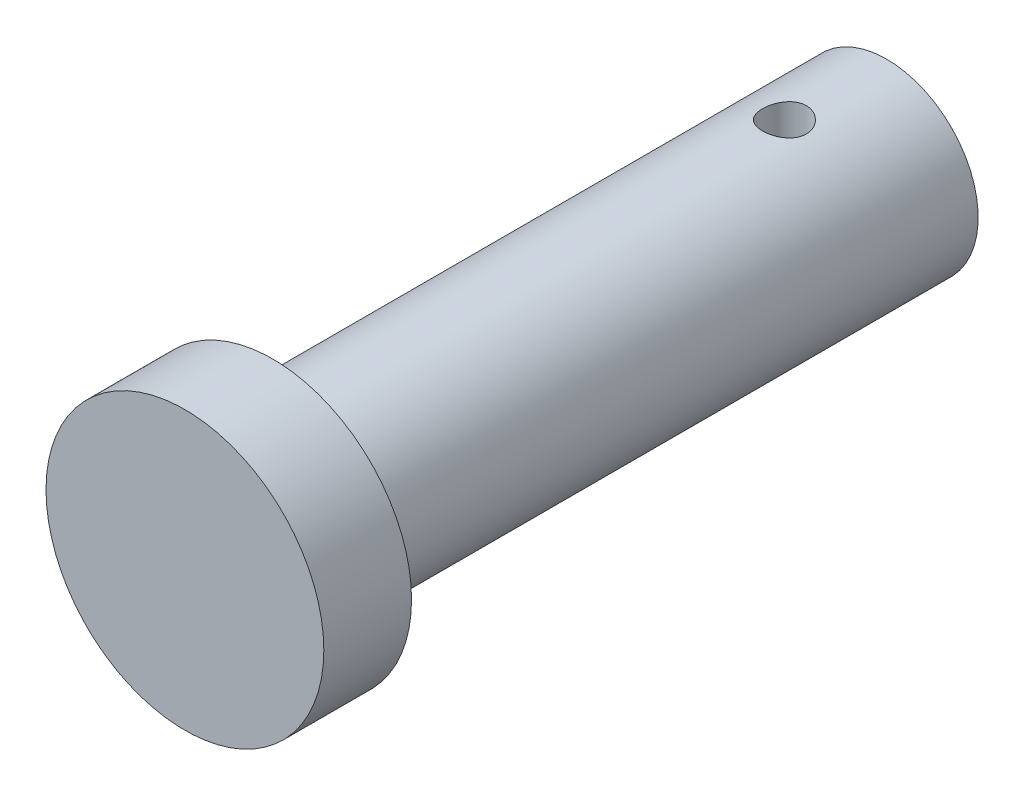
ISO-10303-21;
HEADER;
FILE_DESCRIPTION(('STEP AP214'),'2;1');
FILE_NAME('part.step','',(''),(''),'','','');
FILE_SCHEMA(('AUTOMOTIVE_DESIGN { 1 0 10303 214 1 1 1 1 }'));
ENDSEC;
DATA;
#1=APPLICATION_CONTEXT('core data for automotive mechanical design processes');
#2=APPLICATION_PROTOCOL_DEFINITION('international standard','automotive_design',2000,#1);
#3=PRODUCT_CONTEXT('',#1,'mechanical');
#4=PRODUCT('Part','Part','',(#3));
#5=PRODUCT_RELATED_PRODUCT_CATEGORY('part','',(#4));
#6=PRODUCT_DEFINITION_FORMATION('','',#4);
#7=PRODUCT_DEFINITION_CONTEXT('part definition',#1,'design');
#8=PRODUCT_DEFINITION('design','',#6,#7);
#9=PRODUCT_DEFINITION_SHAPE('','',#8);
#10=(LENGTH_UNIT() NAMED_UNIT(*) SI_UNIT(.MILLI.,.METRE.));
#11=(NAMED_UNIT(*) PLANE_ANGLE_UNIT() SI_UNIT($,.RADIAN.));
#12=(NAMED_UNIT(*) SI_UNIT($,.STERADIAN.) SOLID_ANGLE_UNIT());
#13=UNCERTAINTY_MEASURE_WITH_UNIT(LENGTH_MEASURE(1.E-05),#10,'distance_accuracy_value','');
#14=(GEOMETRIC_REPRESENTATION_CONTEXT(3) GLOBAL_UNCERTAINTY_ASSIGNED_CONTEXT((#13)) GLOBAL_UNIT_ASSIGNED_CONTEXT((#10,
#11,#12)) REPRESENTATION_CONTEXT('',''));
#15=CARTESIAN_POINT('',(0.,0.,0.));
#16=DIRECTION('',(0.,0.,1.));
#17=DIRECTION('',(1.,0.,0.));
#18=AXIS2_PLACEMENT_3D('',#15,#16,#17);
#19=CARTESIAN_POINT('',(0.,0.,12.));
#20=DIRECTION('',(0.,0.,-1.));
#21=DIRECTION('',(-1.,0.,0.));
#22=AXIS2_PLACEMENT_3D('',#19,#20,#21);
#23=CYLINDRICAL_SURFACE('',#22,19.);
#24=CARTESIAN_POINT('',(0.,0.,12.));
#25=DIRECTION('',(0.,0.,1.));
#26=DIRECTION('',(1.,0.,0.));
#27=AXIS2_PLACEMENT_3D('',#24,#25,#26);
#28=CIRCLE('',#27,19.);
#29=CARTESIAN_POINT('',(19.,0.,12.));
#30=VERTEX_POINT('',#29);
#31=EDGE_CURVE('E47',#30,#30,#28,.T.);
#32=ORIENTED_EDGE('',*,*,#31,.F.);
#33=EDGE_LOOP('',(#32));
#34=FACE_BOUND('',#33,.T.);
#35=CARTESIAN_POINT('',(0.,0.,0.));
#36=DIRECTION('',(0.,0.,1.));
#37=DIRECTION('',(1.,0.,0.));
#38=AXIS2_PLACEMENT_3D('',#35,#36,#37);
#39=CIRCLE('',#38,19.);
#40=CARTESIAN_POINT('',(19.,0.,0.));
#41=VERTEX_POINT('',#40);
#42=EDGE_CURVE('E53',#41,#41,#39,.T.);
#43=ORIENTED_EDGE('',*,*,#42,.T.);
#44=EDGE_LOOP('',(#43));
#45=FACE_BOUND('',#44,.T.);
#46=ADVANCED_FACE('F40',(#34,#45),#23,.T.);
#47=CARTESIAN_POINT('',(0.,0.,12.));
#48=DIRECTION('',(0.,0.,1.));
#49=DIRECTION('',(1.,0.,0.));
#50=AXIS2_PLACEMENT_3D('',#47,#48,#49);
#51=PLANE('',#50);
#52=ORIENTED_EDGE('',*,*,#31,.T.);
#53=EDGE_LOOP('',(#52));
#54=FACE_BOUND('',#53,.T.);
#55=ADVANCED_FACE('F83',(#54),#51,.T.);
#56=CARTESIAN_POINT('',(0.,0.,0.));
#57=DIRECTION('',(0.,0.,1.));
#58=DIRECTION('',(1.,0.,0.));
#59=AXIS2_PLACEMENT_3D('',#56,#57,#58);
#60=PLANE('',#59);
#61=CARTESIAN_POINT('',(0.,0.,0.));
#62=DIRECTION('',(0.,0.,-1.));
#63=DIRECTION('',(-1.,0.,0.));
#64=AXIS2_PLACEMENT_3D('',#61,#62,#63);
#65=CIRCLE('',#64,12.5);
#66=CARTESIAN_POINT('',(-12.5,0.,0.));
#67=VERTEX_POINT('',#66);
#68=EDGE_CURVE('E10',#67,#67,#65,.T.);
#69=ORIENTED_EDGE('',*,*,#68,.F.);
#70=EDGE_LOOP('',(#69));
#71=FACE_BOUND('',#70,.T.);
#72=ORIENTED_EDGE('',*,*,#42,.F.);
#73=EDGE_LOOP('',(#72));
#74=FACE_BOUND('',#73,.T.);
#75=ADVANCED_FACE('F82',(#71,#74),#60,.F.);
#76=CARTESIAN_POINT('',(0.,0.,-84.));
#77=DIRECTION('',(0.,0.,1.));
#78=DIRECTION('',(1.,0.,0.));
#79=AXIS2_PLACEMENT_3D('',#76,#77,#78);
#80=CYLINDRICAL_SURFACE('',#79,12.5);
#81=CARTESIAN_POINT('',(0.,-12.5,-67.));
#82=CARTESIAN_POINT('',(0.165963929028719,-12.4999970714968,-67.0000050240773));
#83=CARTESIAN_POINT('',(0.331985420928071,-12.4966615634859,-67.0138184102361));
#84=CARTESIAN_POINT('',(0.659284290971384,-12.4836783946933,-67.0686327395954));
#85=CARTESIAN_POINT('',(0.820558683214278,-12.4740268462166,-67.1096504279947));
#86=CARTESIAN_POINT('',(1.13358839471402,-12.4494823208195,-67.2174923345044));
#87=CARTESIAN_POINT('',(1.28535442324823,-12.4345953702841,-67.2842868898576));
#88=CARTESIAN_POINT('',(1.57552517879764,-12.4011725442513,-67.4416854364459));
#89=CARTESIAN_POINT('',(1.71392971475167,-12.3826366165873,-67.5322897680773));
#90=CARTESIAN_POINT('',(1.97609263393973,-12.3435386014785,-67.7365641783755));
#91=CARTESIAN_POINT('',(2.0995595210048,-12.3229472454311,-67.8506027810493));
#92=CARTESIAN_POINT('',(2.32581080811943,-12.2822574370147,-68.0977188690646));
#93=CARTESIAN_POINT('',(2.4285930462449,-12.2621590363612,-68.230798342041));
#94=CARTESIAN_POINT('',(2.61189993555015,-12.224437969062,-68.5144458330174));
#95=CARTESIAN_POINT('',(2.69210377047565,-12.2068525815312,-68.6652265837588));
#96=CARTESIAN_POINT('',(2.82591582947333,-12.1765733412448,-68.9786198351285));
#97=CARTESIAN_POINT('',(2.87952794169564,-12.1638787734309,-69.1412306020232));
#98=CARTESIAN_POINT('',(2.95765058108664,-12.1451184675007,-69.4704765732689));
#99=CARTESIAN_POINT('',(2.98268262400617,-12.1389341034343,-69.6369811215255));
#100=CARTESIAN_POINT('',(3.00455808879087,-12.1335389605945,-69.9719323796428));
#101=CARTESIAN_POINT('',(3.001405716824,-12.1343271412568,-70.1403787959569));
#102=CARTESIAN_POINT('',(2.96741912081943,-12.1426811387008,-70.4704759660129));
#103=CARTESIAN_POINT('',(2.93720103400495,-12.1500960921292,-70.6321945651895));
#104=CARTESIAN_POINT('',(2.85092141637189,-12.1706283738785,-70.9481973166478));
#105=CARTESIAN_POINT('',(2.79485817372028,-12.1837460799133,-71.1024809757344));
#106=CARTESIAN_POINT('',(2.65794121231782,-12.2143476734445,-71.4009129780844));
#107=CARTESIAN_POINT('',(2.5768594824696,-12.2318714325758,-71.5449524529167));
#108=CARTESIAN_POINT('',(2.39236688956382,-12.2692875046197,-71.8176045007226));
#109=CARTESIAN_POINT('',(2.28895240342647,-12.2891802016137,-71.9462145652851));
#110=CARTESIAN_POINT('',(2.05951493908847,-12.329732025739,-72.1878935703187));
#111=CARTESIAN_POINT('',(1.93297064389908,-12.3503975788014,-72.3004670990622));
#112=CARTESIAN_POINT('',(1.66255592459692,-12.3896951594929,-72.5028847197464));
#113=CARTESIAN_POINT('',(1.51868504982141,-12.4083271342049,-72.5927282202926));
#114=CARTESIAN_POINT('',(1.21702847718581,-12.4415394956922,-72.7472972206128));
#115=CARTESIAN_POINT('',(1.05920278696055,-12.4561077058019,-72.8119474562378));
#116=CARTESIAN_POINT('',(0.734497606078676,-12.4794620474154,-72.9136650790486));
#117=CARTESIAN_POINT('',(0.56761971338766,-12.4882491958651,-72.9507373176268));
#118=CARTESIAN_POINT('',(0.233787399651661,-12.4989027542709,-72.9955020646521));
#119=CARTESIAN_POINT('',(0.0669284805450053,-12.5009282130753,-73.0038698924616));
#120=CARTESIAN_POINT('',(-0.26580438158663,-12.4982807419474,-72.9928332331491));
#121=CARTESIAN_POINT('',(-0.431678404764951,-12.4936083648176,-72.9734310380128));
#122=CARTESIAN_POINT('',(-0.755422580108846,-12.4781916395217,-72.9079630214836));
#123=CARTESIAN_POINT('',(-0.913370579311304,-12.4675301590363,-72.8622608904262));
#124=CARTESIAN_POINT('',(-1.21935330013476,-12.4413335015664,-72.7459018083048));
#125=CARTESIAN_POINT('',(-1.3673870666415,-12.4257978558334,-72.6752424570219));
#126=CARTESIAN_POINT('',(-1.6520615099557,-12.3911910149582,-72.5096334064021));
#127=CARTESIAN_POINT('',(-1.78847176740356,-12.3720653178033,-72.4142992830756));
#128=CARTESIAN_POINT('',(-2.04359904096633,-12.3324936406987,-72.2025430709866));
#129=CARTESIAN_POINT('',(-2.16231325074337,-12.3120474520734,-72.0861176439192));
#130=CARTESIAN_POINT('',(-2.38142453789941,-12.2715742142771,-71.8323591687915));
#131=CARTESIAN_POINT('',(-2.48134974047369,-12.2515669262668,-71.6946148779179));
#132=CARTESIAN_POINT('',(-2.65666020824081,-12.2147538797452,-71.4039095721033));
#133=CARTESIAN_POINT('',(-2.7320465722335,-12.1979479778962,-71.2509492389065));
#134=CARTESIAN_POINT('',(-2.85558993518171,-12.1696189519335,-70.934987486456));
#135=CARTESIAN_POINT('',(-2.90390754385905,-12.1580647463107,-70.7720517965788));
#136=CARTESIAN_POINT('',(-2.97238380283979,-12.1415072663683,-70.4400538149793));
#137=CARTESIAN_POINT('',(-2.99254804274991,-12.1365026916888,-70.2709927462382));
#138=CARTESIAN_POINT('',(-3.00387066449353,-12.1337046220624,-69.9363292997194));
#139=CARTESIAN_POINT('',(-2.99578106592266,-12.1357241633848,-69.7707535036733));
#140=CARTESIAN_POINT('',(-2.95253345626267,-12.1463176460425,-69.4434002357763));
#141=CARTESIAN_POINT('',(-2.91737590900096,-12.1548914750658,-69.2816226988886));
#142=CARTESIAN_POINT('',(-2.82138591303537,-12.1775274976748,-68.9672024474518));
#143=CARTESIAN_POINT('',(-2.76068402045611,-12.191561756094,-68.8145177274163));
#144=CARTESIAN_POINT('',(-2.61543373580582,-12.2235433612686,-68.5213955861163));
#145=CARTESIAN_POINT('',(-2.53088229934855,-12.2414912075257,-68.3809597314136));
#146=CARTESIAN_POINT('',(-2.33793007708463,-12.279819325529,-68.1126629998805));
#147=CARTESIAN_POINT('',(-2.22900267979018,-12.3002478697533,-67.9851876769013));
#148=CARTESIAN_POINT('',(-1.99143074773236,-12.3409359831145,-67.7500800119481));
#149=CARTESIAN_POINT('',(-1.86278158874233,-12.361195511444,-67.6424523367898));
#150=CARTESIAN_POINT('',(-1.58688299880139,-12.3996570299581,-67.4483907404453));
#151=CARTESIAN_POINT('',(-1.43936414359401,-12.4178200201219,-67.362331594558));
#152=CARTESIAN_POINT('',(-1.13153622828567,-12.4496380610582,-67.2163704672521));
#153=CARTESIAN_POINT('',(-0.971236973691219,-12.4632965272855,-67.1564486566084));
#154=CARTESIAN_POINT('',(-0.675887025694763,-12.4824059901497,-67.0739613748622));
#155=CARTESIAN_POINT('',(-0.542312066268418,-12.4889599449579,-67.0462833842143));
#156=CARTESIAN_POINT('',(-0.272504227478245,-12.4977580149525,-67.0093012191481));
#157=CARTESIAN_POINT('',(-0.136271517915773,-12.5000024045682,-66.9999958747745));
#158=CARTESIAN_POINT('',(0.,-12.5,-67.));
#159=B_SPLINE_CURVE_WITH_KNOTS('',3,(#81,#82,#83,#84,#85,#86,#87,#88,#89,#90,#91,#92,#93,#94,
#95,#96,#97,#98,#99,#100,#101,#102,#103,#104,#105,#106,#107,#108,#109,#110,#111,#112,#113,#114,
#115,#116,#117,#118,#119,#120,#121,#122,#123,#124,#125,#126,#127,#128,#129,#130,#131,#132,#133,
#134,#135,#136,#137,#138,#139,#140,#141,#142,#143,#144,#145,#146,#147,#148,#149,#150,#151,#152,
#153,#154,#155,#156,#157,#158),.UNSPECIFIED.,.T.,.F.,(4,2,2,2,2,2,2,2,2,2,2,2,2,2,2,2,2,2,2,2,2,
2,2,2,2,2,2,2,2,2,2,2,2,2,2,2,2,2,4),(0.,0.497392599366679,0.995091645758826,1.49221966408501,
1.9893547899852,2.49500570148357,3.00070943533306,3.51327262050848,4.02576083835037,
4.52873995359112,5.03164400680464,5.52338274964838,6.01515406709139,6.51154667521173,
7.00801987450004,7.51749958381935,8.02699254752171,8.53799614678204,9.04890983140416,
9.54771776810827,10.0464845383097,10.5385143736981,11.0305915421211,11.5308523313794,
12.0311923705731,12.5427824523192,13.0543496229378,13.5628484119093,14.0712462285019,
14.5662165454702,15.0611783809799,15.5536406351284,16.0461657803879,16.5505844610431,
17.055121595827,17.5678974206352,18.0802835459069,18.4887142303991,18.897118905514),.UNSPECIFIED.);
#160=CARTESIAN_POINT('',(0.,-12.5,-67.));
#161=VERTEX_POINT('',#160);
#162=EDGE_CURVE('E37',#161,#161,#159,.T.);
#163=ORIENTED_EDGE('',*,*,#162,.T.);
#164=EDGE_LOOP('',(#163));
#165=FACE_BOUND('',#164,.T.);
#166=CARTESIAN_POINT('',(0.,12.5,-67.));
#167=CARTESIAN_POINT('',(-0.165963929028713,12.4999970714968,-67.0000050240773));
#168=CARTESIAN_POINT('',(-0.331985420928065,12.4966615634859,-67.0138184102361));
#169=CARTESIAN_POINT('',(-0.659284290971378,12.4836783946932,-67.0686327395954));
#170=CARTESIAN_POINT('',(-0.820558683214273,12.4740268462166,-67.1096504279947));
#171=CARTESIAN_POINT('',(-1.13358839471402,12.4494823208195,-67.2174923345044));
#172=CARTESIAN_POINT('',(-1.28535442324822,12.4345953702841,-67.2842868898576));
#173=CARTESIAN_POINT('',(-1.57552517879763,12.4011725442513,-67.4416854364459));
#174=CARTESIAN_POINT('',(-1.71392971475166,12.3826366165873,-67.5322897680773));
#175=CARTESIAN_POINT('',(-1.97609263393972,12.3435386014785,-67.7365641783755));
#176=CARTESIAN_POINT('',(-2.0995595210048,12.3229472454311,-67.8506027810493));
#177=CARTESIAN_POINT('',(-2.32581080811943,12.2822574370147,-68.0977188690646));
#178=CARTESIAN_POINT('',(-2.42859304624489,12.2621590363612,-68.230798342041));
#179=CARTESIAN_POINT('',(-2.61189993555015,12.224437969062,-68.5144458330175));
#180=CARTESIAN_POINT('',(-2.69210377047565,12.2068525815312,-68.6652265837589));
#181=CARTESIAN_POINT('',(-2.82591582947333,12.1765733412448,-68.9786198351285));
#182=CARTESIAN_POINT('',(-2.87952794169564,12.1638787734309,-69.1412306020232));
#183=CARTESIAN_POINT('',(-2.95765058108663,12.1451184675007,-69.4704765732689));
#184=CARTESIAN_POINT('',(-2.98268262400616,12.1389341034343,-69.6369811215255));
#185=CARTESIAN_POINT('',(-3.00455808879087,12.1335389605945,-69.9719323796428));
#186=CARTESIAN_POINT('',(-3.00140571682399,12.1343271412568,-70.1403787959569));
#187=CARTESIAN_POINT('',(-2.96741912081942,12.1426811387008,-70.4704759660129));
#188=CARTESIAN_POINT('',(-2.93720103400494,12.1500960921292,-70.6321945651895));
#189=CARTESIAN_POINT('',(-2.85092141637189,12.1706283738785,-70.9481973166478));
#190=CARTESIAN_POINT('',(-2.79485817372027,12.1837460799133,-71.1024809757344));
#191=CARTESIAN_POINT('',(-2.65794121231781,12.2143476734445,-71.4009129780844));
#192=CARTESIAN_POINT('',(-2.57685948246959,12.2318714325758,-71.5449524529167));
#193=CARTESIAN_POINT('',(-2.39236688956382,12.2692875046197,-71.8176045007226));
#194=CARTESIAN_POINT('',(-2.28895240342646,12.2891802016137,-71.9462145652851));
#195=CARTESIAN_POINT('',(-2.05951493908846,12.329732025739,-72.1878935703187));
#196=CARTESIAN_POINT('',(-1.93297064389908,12.3503975788014,-72.3004670990622));
#197=CARTESIAN_POINT('',(-1.66255592459691,12.3896951594929,-72.5028847197464));
#198=CARTESIAN_POINT('',(-1.5186850498214,12.4083271342049,-72.5927282202926));
#199=CARTESIAN_POINT('',(-1.21702847718581,12.4415394956922,-72.7472972206128));
#200=CARTESIAN_POINT('',(-1.05920278696054,12.4561077058019,-72.8119474562378));
#201=CARTESIAN_POINT('',(-0.734497606078672,12.4794620474154,-72.9136650790486));
#202=CARTESIAN_POINT('',(-0.567619713387655,12.4882491958651,-72.9507373176268));
#203=CARTESIAN_POINT('',(-0.233787399651657,12.4989027542709,-72.9955020646521));
#204=CARTESIAN_POINT('',(-0.0669284805450011,12.5009282130753,-73.0038698924616));
#205=CARTESIAN_POINT('',(0.265804381586634,12.4982807419474,-72.9928332331491));
#206=CARTESIAN_POINT('',(0.431678404764957,12.4936083648176,-72.9734310380128));
#207=CARTESIAN_POINT('',(0.75542258010885,12.4781916395217,-72.9079630214836));
#208=CARTESIAN_POINT('',(0.913370579311307,12.4675301590363,-72.8622608904262));
#209=CARTESIAN_POINT('',(1.21935330013476,12.4413335015664,-72.7459018083048));
#210=CARTESIAN_POINT('',(1.3673870666415,12.4257978558334,-72.6752424570219));
#211=CARTESIAN_POINT('',(1.65206150995571,12.3911910149582,-72.5096334064021));
#212=CARTESIAN_POINT('',(1.78847176740356,12.3720653178033,-72.4142992830756));
#213=CARTESIAN_POINT('',(2.04359904096634,12.3324936406987,-72.2025430709866));
#214=CARTESIAN_POINT('',(2.16231325074337,12.3120474520734,-72.0861176439192));
#215=CARTESIAN_POINT('',(2.38142453789941,12.2715742142771,-71.8323591687915));
#216=CARTESIAN_POINT('',(2.4813497404737,12.2515669262668,-71.6946148779179));
#217=CARTESIAN_POINT('',(2.65666020824082,12.2147538797452,-71.4039095721033));
#218=CARTESIAN_POINT('',(2.7320465722335,12.1979479778962,-71.2509492389065));
#219=CARTESIAN_POINT('',(2.85558993518172,12.1696189519335,-70.934987486456));
#220=CARTESIAN_POINT('',(2.90390754385905,12.1580647463107,-70.7720517965788));
#221=CARTESIAN_POINT('',(2.97238380283979,12.1415072663683,-70.4400538149793));
#222=CARTESIAN_POINT('',(2.99254804274991,12.1365026916888,-70.2709927462382));
#223=CARTESIAN_POINT('',(3.00387066449354,12.1337046220624,-69.9363292997194));
#224=CARTESIAN_POINT('',(2.99578106592266,12.1357241633848,-69.7707535036733));
#225=CARTESIAN_POINT('',(2.95253345626268,12.1463176460425,-69.4434002357763));
#226=CARTESIAN_POINT('',(2.91737590900097,12.1548914750658,-69.2816226988886));
#227=CARTESIAN_POINT('',(2.82138591303538,12.1775274976748,-68.9672024474518));
#228=CARTESIAN_POINT('',(2.76068402045612,12.191561756094,-68.8145177274163));
#229=CARTESIAN_POINT('',(2.61543373580584,12.2235433612686,-68.5213955861163));
#230=CARTESIAN_POINT('',(2.53088229934856,12.2414912075257,-68.3809597314137));
#231=CARTESIAN_POINT('',(2.33793007708465,12.279819325529,-68.1126629998805));
#232=CARTESIAN_POINT('',(2.2290026797902,12.3002478697533,-67.9851876769013));
#233=CARTESIAN_POINT('',(1.99143074773238,12.3409359831145,-67.7500800119481));
#234=CARTESIAN_POINT('',(1.86278158874235,12.361195511444,-67.6424523367898));
#235=CARTESIAN_POINT('',(1.58688299880141,12.3996570299581,-67.4483907404453));
#236=CARTESIAN_POINT('',(1.43936414359403,12.4178200201219,-67.362331594558));
#237=CARTESIAN_POINT('',(1.13153622828568,12.4496380610582,-67.2163704672521));
#238=CARTESIAN_POINT('',(0.971236973691228,12.4632965272855,-67.1564486566084));
#239=CARTESIAN_POINT('',(0.675887025694771,12.4824059901497,-67.0739613748622));
#240=CARTESIAN_POINT('',(0.542312066268425,12.4889599449579,-67.0462833842143));
#241=CARTESIAN_POINT('',(0.272504227478252,12.4977580149525,-67.0093012191481));
#242=CARTESIAN_POINT('',(0.13627151791578,12.5000024045682,-66.9999958747745));
#243=CARTESIAN_POINT('',(0.,12.5,-67.));
#244=B_SPLINE_CURVE_WITH_KNOTS('',3,(#166,#167,#168,#169,#170,#171,#172,#173,#174,#175,#176,
#177,#178,#179,#180,#181,#182,#183,#184,#185,#186,#187,#188,#189,#190,#191,#192,#193,#194,#195,
#196,#197,#198,#199,#200,#201,#202,#203,#204,#205,#206,#207,#208,#209,#210,#211,#212,#213,#214,
#215,#216,#217,#218,#219,#220,#221,#222,#223,#224,#225,#226,#227,#228,#229,#230,#231,#232,#233,
#234,#235,#236,#237,#238,#239,#240,#241,#242,#243),.UNSPECIFIED.,.T.,.F.,(4,2,2,2,2,2,2,2,2,2,2,
2,2,2,2,2,2,2,2,2,2,2,2,2,2,2,2,2,2,2,2,2,2,2,2,2,2,2,4),(0.,0.497392599366679,
0.995091645758827,1.49221966408501,1.9893547899852,2.49500570148358,3.00070943533306,
3.5132726205085,4.02576083835038,4.52873995359112,5.03164400680464,5.52338274964838,
6.01515406709139,6.51154667521173,7.00801987450004,7.51749958381935,8.02699254752171,
8.53799614678204,9.04890983140416,9.54771776810827,10.0464845383097,10.5385143736981,
11.0305915421211,11.5308523313794,12.0311923705731,12.5427824523192,13.0543496229378,
13.5628484119093,14.0712462285019,14.5662165454702,15.0611783809799,15.5536406351284,
16.0461657803879,16.5505844610431,17.0551215958269,17.5678974206352,18.0802835459069,
18.4887142303991,18.897118905514),.UNSPECIFIED.);
#245=CARTESIAN_POINT('',(0.,12.5,-67.));
#246=VERTEX_POINT('',#245);
#247=EDGE_CURVE('E58',#246,#246,#244,.T.);
#248=ORIENTED_EDGE('',*,*,#247,.T.);
#249=EDGE_LOOP('',(#248));
#250=FACE_BOUND('',#249,.T.);
#251=CARTESIAN_POINT('',(0.,0.,-84.));
#252=DIRECTION('',(0.,0.,-1.));
#253=DIRECTION('',(-1.,0.,0.));
#254=AXIS2_PLACEMENT_3D('',#251,#252,#253);
#255=CIRCLE('',#254,12.5);
#256=CARTESIAN_POINT('',(-12.5,0.,-84.));
#257=VERTEX_POINT('',#256);
#258=EDGE_CURVE('E60',#257,#257,#255,.T.);
#259=ORIENTED_EDGE('',*,*,#258,.F.);
#260=EDGE_LOOP('',(#259));
#261=FACE_BOUND('',#260,.T.);
#262=ORIENTED_EDGE('',*,*,#68,.T.);
#263=EDGE_LOOP('',(#262));
#264=FACE_BOUND('',#263,.T.);
#265=ADVANCED_FACE('F64',(#165,#250,#261,#264),#80,.T.);
#266=CARTESIAN_POINT('',(0.,0.,-84.));
#267=DIRECTION('',(0.,0.,-1.));
#268=DIRECTION('',(-1.,0.,0.));
#269=AXIS2_PLACEMENT_3D('',#266,#267,#268);
#270=PLANE('',#269);
#271=ORIENTED_EDGE('',*,*,#258,.T.);
#272=EDGE_LOOP('',(#271));
#273=FACE_BOUND('',#272,.T.);
#274=ADVANCED_FACE('F75',(#273),#270,.T.);
#275=CARTESIAN_POINT('',(0.,-42.,-70.));
#276=DIRECTION('',(0.,1.,0.));
#277=DIRECTION('',(0.,0.,1.));
#278=AXIS2_PLACEMENT_3D('',#275,#276,#277);
#279=CYLINDRICAL_SURFACE('',#278,3.);
#280=ORIENTED_EDGE('',*,*,#247,.F.);
#281=EDGE_LOOP('',(#280));
#282=FACE_BOUND('',#281,.T.);
#283=ORIENTED_EDGE('',*,*,#162,.F.);
#284=EDGE_LOOP('',(#283));
#285=FACE_BOUND('',#284,.T.);
#286=ADVANCED_FACE('F66',(#282,#285),#279,.F.);
#287=CLOSED_SHELL('',(#46,#55,#75,#265,#274,#286));
#288=MANIFOLD_SOLID_BREP('B2',#287);
#289=ADVANCED_BREP_SHAPE_REPRESENTATION('',(#18,#288),#14);
#290=SHAPE_DEFINITION_REPRESENTATION(#9,#289);
ENDSEC;
END-ISO-10303-21;
